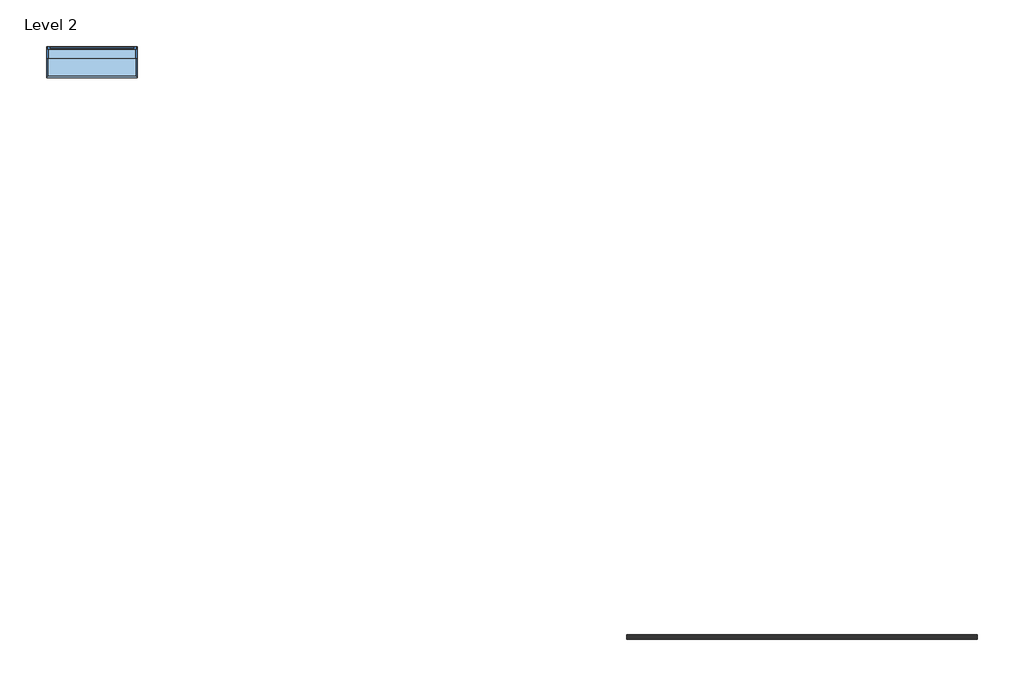
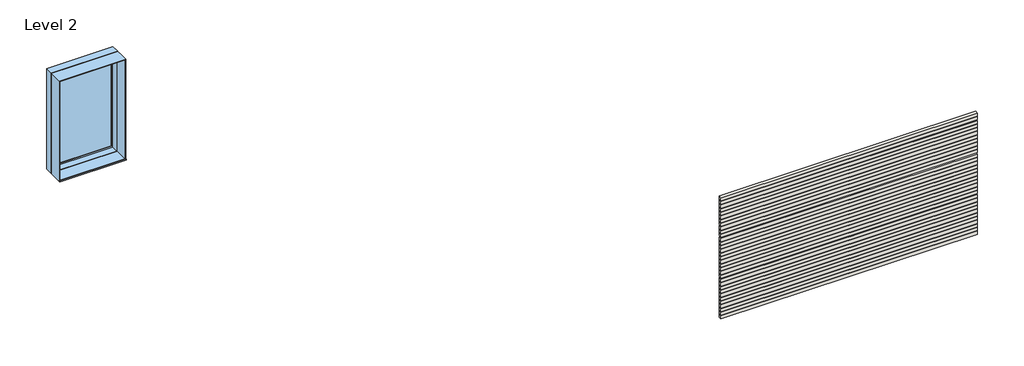
# One storey: 3 walls, 1 window.
"""IFC4 building model written with IfcOpenShell, lengths in millimetres."""

from ifc_helpers import new_model, si_unit, frame, origin, place, context, project, spatial, polyline, outline, extrude, transform, mapped, element, save
from components import window_e9f06afb

model = new_model("IFC4")

# Units and contexts
model_context = context("Model", 3, world=origin())
ifc_project = project(units=[si_unit("LENGTHUNIT", "METRE", prefix="MILLI")], contexts=[model_context])

# Site, building, storey
site = spatial("IfcSite", under=ifc_project)
building = spatial("IfcBuilding", under=site)
storey = spatial("IfcBuildingStorey", under=building, Name="Level 2", Elevation=3048.0)

# Walls
placement = place(None, origin())
element("IfcWall", 1, ObjectType="Generic - 3\" white 2", at=placement, inside=storey, context=model_context, shape_type="SweptSolid", body=[
    extrude(outline(polyline([(7352.8964234, 5106.5999244), (1468.8829427, 5106.5999244), (1468.8829427, 5182.7999244), (7352.8964234, 5182.7999244), (7352.8964234, 5106.5999244)])), frame((0.0, 0.0, 1971.675), z_axis=(0.0, 0.0, 1.0), x_axis=(1.0, 0.0, 0.0)), (0.0, 0.0, 1.0), 76.2),
    extrude(outline(polyline([(7352.8964234, 5106.5999244), (1468.8829427, 5106.5999244), (1468.8829427, 5182.7999244), (7352.8964234, 5182.7999244), (7352.8964234, 5106.5999244)])), frame((0.0, 0.0, 2060.575), z_axis=(0.0, 0.0, 1.0), x_axis=(1.0, 0.0, 0.0)), (0.0, 0.0, 1.0), 76.2),
    extrude(outline(polyline([(7352.8964234, 5106.5999244), (1468.8829427, 5106.5999244), (1468.8829427, 5182.7999244), (7352.8964234, 5182.7999244), (7352.8964234, 5106.5999244)])), frame((0.0, 0.0, 2149.475), z_axis=(0.0, 0.0, 1.0), x_axis=(1.0, 0.0, 0.0)), (0.0, 0.0, 1.0), 76.2),
    extrude(outline(polyline([(7352.8964234, 5106.5999244), (1468.8829427, 5106.5999244), (1468.8829427, 5182.7999244), (7352.8964234, 5182.7999244), (7352.8964234, 5106.5999244)])), frame((0.0, 0.0, 2238.375), z_axis=(0.0, 0.0, 1.0), x_axis=(1.0, 0.0, 0.0)), (0.0, 0.0, 1.0), 76.2),
    extrude(outline(polyline([(7352.8964234, 5106.5999244), (1468.8829427, 5106.5999244), (1468.8829427, 5182.7999244), (7352.8964234, 5182.7999244), (7352.8964234, 5106.5999244)])), frame((0.0, 0.0, 2327.275), z_axis=(0.0, 0.0, 1.0), x_axis=(1.0, 0.0, 0.0)), (0.0, 0.0, 1.0), 76.2),
    extrude(outline(polyline([(7352.8964234, 5106.5999244), (1468.8829427, 5106.5999244), (1468.8829427, 5182.7999244), (7352.8964234, 5182.7999244), (7352.8964234, 5106.5999244)])), frame((0.0, 0.0, 2416.175), z_axis=(0.0, 0.0, 1.0), x_axis=(1.0, 0.0, 0.0)), (0.0, 0.0, 1.0), 76.2),
    extrude(outline(polyline([(7352.8964234, 5106.5999244), (1468.8829427, 5106.5999244), (1468.8829427, 5182.7999244), (7352.8964234, 5182.7999244), (7352.8964234, 5106.5999244)])), frame((0.0, 0.0, 2505.075), z_axis=(0.0, 0.0, 1.0), x_axis=(1.0, 0.0, 0.0)), (0.0, 0.0, 1.0), 76.2),
    extrude(outline(polyline([(7352.8964234, 5106.5999244), (1468.8829427, 5106.5999244), (1468.8829427, 5182.7999244), (7352.8964234, 5182.7999244), (7352.8964234, 5106.5999244)])), frame((0.0, 0.0, 2593.975), z_axis=(0.0, 0.0, 1.0), x_axis=(1.0, 0.0, 0.0)), (0.0, 0.0, 1.0), 76.2),
    extrude(outline(polyline([(7352.8964234, 5106.5999244), (1468.8829427, 5106.5999244), (1468.8829427, 5182.7999244), (7352.8964234, 5182.7999244), (7352.8964234, 5106.5999244)])), frame((0.0, 0.0, 2682.875), z_axis=(0.0, 0.0, 1.0), x_axis=(1.0, 0.0, 0.0)), (0.0, 0.0, 1.0), 76.2),
    extrude(outline(polyline([(7352.8964234, 5106.5999244), (1468.8829427, 5106.5999244), (1468.8829427, 5182.7999244), (7352.8964234, 5182.7999244), (7352.8964234, 5106.5999244)])), frame((0.0, 0.0, 2771.775), z_axis=(0.0, 0.0, 1.0), x_axis=(1.0, 0.0, 0.0)), (0.0, 0.0, 1.0), 76.2),
    extrude(outline(polyline([(7352.8964234, 5106.5999244), (1468.8829427, 5106.5999244), (1468.8829427, 5182.7999244), (7352.8964234, 5182.7999244), (7352.8964234, 5106.5999244)])), frame((0.0, 0.0, 2860.675), z_axis=(0.0, 0.0, 1.0), x_axis=(1.0, 0.0, 0.0)), (0.0, 0.0, 1.0), 76.2),
])
element("IfcWall", 2, ObjectType="Generic - 3\" white 2", at=placement, inside=storey, context=model_context, shape_type="SweptSolid", body=[
    extrude(outline(polyline([(7352.8964234, 5106.5999244), (1468.8829427, 5106.5999244), (1468.8829427, 5182.7999244), (7352.8964234, 5182.7999244), (7352.8964234, 5106.5999244)])), frame((0.0, 0.0, 2959.1), z_axis=(0.0, 0.0, 1.0), x_axis=(1.0, 0.0, 0.0)), (0.0, 0.0, 1.0), 76.2),
    extrude(outline(polyline([(7352.8964234, 5106.5999244), (1468.8829427, 5106.5999244), (1468.8829427, 5182.7999244), (7352.8964234, 5182.7999244), (7352.8964234, 5106.5999244)])), frame((0.0, 0.0, 3048.0), z_axis=(0.0, 0.0, 1.0), x_axis=(1.0, 0.0, 0.0)), (0.0, 0.0, 1.0), 76.2),
    extrude(outline(polyline([(7352.8964234, 5106.5999244), (1468.8829427, 5106.5999244), (1468.8829427, 5182.7999244), (7352.8964234, 5182.7999244), (7352.8964234, 5106.5999244)])), frame((0.0, 0.0, 3136.9), z_axis=(0.0, 0.0, 1.0), x_axis=(1.0, 0.0, 0.0)), (0.0, 0.0, 1.0), 76.2),
    extrude(outline(polyline([(7352.8964234, 5106.5999244), (1468.8829427, 5106.5999244), (1468.8829427, 5182.7999244), (7352.8964234, 5182.7999244), (7352.8964234, 5106.5999244)])), frame((0.0, 0.0, 3225.8), z_axis=(0.0, 0.0, 1.0), x_axis=(1.0, 0.0, 0.0)), (0.0, 0.0, 1.0), 76.2),
    extrude(outline(polyline([(7352.8964234, 5106.5999244), (1468.8829427, 5106.5999244), (1468.8829427, 5182.7999244), (7352.8964234, 5182.7999244), (7352.8964234, 5106.5999244)])), frame((0.0, 0.0, 3314.7), z_axis=(0.0, 0.0, 1.0), x_axis=(1.0, 0.0, 0.0)), (0.0, 0.0, 1.0), 76.2),
    extrude(outline(polyline([(7352.8964234, 5106.5999244), (1468.8829427, 5106.5999244), (1468.8829427, 5182.7999244), (7352.8964234, 5182.7999244), (7352.8964234, 5106.5999244)])), frame((0.0, 0.0, 3403.6), z_axis=(0.0, 0.0, 1.0), x_axis=(1.0, 0.0, 0.0)), (0.0, 0.0, 1.0), 76.2),
    extrude(outline(polyline([(7352.8964234, 5106.5999244), (1468.8829427, 5106.5999244), (1468.8829427, 5182.7999244), (7352.8964234, 5182.7999244), (7352.8964234, 5106.5999244)])), frame((0.0, 0.0, 3492.5), z_axis=(0.0, 0.0, 1.0), x_axis=(1.0, 0.0, 0.0)), (0.0, 0.0, 1.0), 76.2),
    extrude(outline(polyline([(7352.8964234, 5106.5999244), (1468.8829427, 5106.5999244), (1468.8829427, 5182.7999244), (7352.8964234, 5182.7999244), (7352.8964234, 5106.5999244)])), frame((0.0, 0.0, 3581.4), z_axis=(0.0, 0.0, 1.0), x_axis=(1.0, 0.0, 0.0)), (0.0, 0.0, 1.0), 76.2),
    extrude(outline(polyline([(7352.8964234, 5106.5999244), (1468.8829427, 5106.5999244), (1468.8829427, 5182.7999244), (7352.8964234, 5182.7999244), (7352.8964234, 5106.5999244)])), frame((0.0, 0.0, 3670.3), z_axis=(0.0, 0.0, 1.0), x_axis=(1.0, 0.0, 0.0)), (0.0, 0.0, 1.0), 76.2),
    extrude(outline(polyline([(7352.8964234, 5106.5999244), (1468.8829427, 5106.5999244), (1468.8829427, 5182.7999244), (7352.8964234, 5182.7999244), (7352.8964234, 5106.5999244)])), frame((0.0, 0.0, 3759.2), z_axis=(0.0, 0.0, 1.0), x_axis=(1.0, 0.0, 0.0)), (0.0, 0.0, 1.0), 76.2),
    extrude(outline(polyline([(7352.8964234, 5106.5999244), (1468.8829427, 5106.5999244), (1468.8829427, 5182.7999244), (7352.8964234, 5182.7999244), (7352.8964234, 5106.5999244)])), frame((0.0, 0.0, 3848.1), z_axis=(0.0, 0.0, 1.0), x_axis=(1.0, 0.0, 0.0)), (0.0, 0.0, 1.0), 76.2),
])
element("IfcWall", 3, ObjectType="Generic - 3\" white 2", at=placement, inside=storey, context=model_context, shape_type="SweptSolid", body=[
    extrude(outline(polyline([(7352.8964234, 5106.5999244), (1468.8829427, 5106.5999244), (1468.8829427, 5182.7999244), (7352.8964234, 5182.7999244), (7352.8964234, 5106.5999244)])), frame((0.0, 0.0, 3950.7840126), z_axis=(0.0, 0.0, 1.0), x_axis=(1.0, 0.0, 0.0)), (0.0, 0.0, 1.0), 76.2),
    extrude(outline(polyline([(7352.8964234, 5106.5999244), (1468.8829427, 5106.5999244), (1468.8829427, 5182.7999244), (7352.8964234, 5182.7999244), (7352.8964234, 5106.5999244)])), frame((0.0, 0.0, 4039.6840126), z_axis=(0.0, 0.0, 1.0), x_axis=(1.0, 0.0, 0.0)), (0.0, 0.0, 1.0), 76.2),
    extrude(outline(polyline([(7352.8964234, 5106.5999244), (1468.8829427, 5106.5999244), (1468.8829427, 5182.7999244), (7352.8964234, 5182.7999244), (7352.8964234, 5106.5999244)])), frame((0.0, 0.0, 4128.5840126), z_axis=(0.0, 0.0, 1.0), x_axis=(1.0, 0.0, 0.0)), (0.0, 0.0, 1.0), 76.2),
    extrude(outline(polyline([(7352.8964234, 5106.5999244), (1468.8829427, 5106.5999244), (1468.8829427, 5182.7999244), (7352.8964234, 5182.7999244), (7352.8964234, 5106.5999244)])), frame((0.0, 0.0, 4217.4840126), z_axis=(0.0, 0.0, 1.0), x_axis=(1.0, 0.0, 0.0)), (0.0, 0.0, 1.0), 76.2),
    extrude(outline(polyline([(7352.8964234, 5106.5999244), (1468.8829427, 5106.5999244), (1468.8829427, 5182.7999244), (7352.8964234, 5182.7999244), (7352.8964234, 5106.5999244)])), frame((0.0, 0.0, 4306.3840126), z_axis=(0.0, 0.0, 1.0), x_axis=(1.0, 0.0, 0.0)), (0.0, 0.0, 1.0), 76.2),
    extrude(outline(polyline([(7352.8964234, 5106.5999244), (1468.8829427, 5106.5999244), (1468.8829427, 5182.7999244), (7352.8964234, 5182.7999244), (7352.8964234, 5106.5999244)])), frame((0.0, 0.0, 4395.2840126), z_axis=(0.0, 0.0, 1.0), x_axis=(1.0, 0.0, 0.0)), (0.0, 0.0, 1.0), 76.2),
    extrude(outline(polyline([(7352.8964234, 5106.5999244), (1468.8829427, 5106.5999244), (1468.8829427, 5182.7999244), (7352.8964234, 5182.7999244), (7352.8964234, 5106.5999244)])), frame((0.0, 0.0, 4484.1840126), z_axis=(0.0, 0.0, 1.0), x_axis=(1.0, 0.0, 0.0)), (0.0, 0.0, 1.0), 76.2),
    extrude(outline(polyline([(7352.8964234, 5106.5999244), (1468.8829427, 5106.5999244), (1468.8829427, 5182.7999244), (7352.8964234, 5182.7999244), (7352.8964234, 5106.5999244)])), frame((0.0, 0.0, 4573.0840126), z_axis=(0.0, 0.0, 1.0), x_axis=(1.0, 0.0, 0.0)), (0.0, 0.0, 1.0), 76.2),
    extrude(outline(polyline([(7352.8964234, 5106.5999244), (1468.8829427, 5106.5999244), (1468.8829427, 5182.7999244), (7352.8964234, 5182.7999244), (7352.8964234, 5106.5999244)])), frame((0.0, 0.0, 4661.9840126), z_axis=(0.0, 0.0, 1.0), x_axis=(1.0, 0.0, 0.0)), (0.0, 0.0, 1.0), 76.2),
    extrude(outline(polyline([(7352.8964234, 5106.5999244), (1468.8829427, 5106.5999244), (1468.8829427, 5182.7999244), (7352.8964234, 5182.7999244), (7352.8964234, 5106.5999244)])), frame((0.0, 0.0, 4750.8840126), z_axis=(0.0, 0.0, 1.0), x_axis=(1.0, 0.0, 0.0)), (0.0, 0.0, 1.0), 76.2),
    extrude(outline(polyline([(7352.8964234, 5106.5999244), (1468.8829427, 5106.5999244), (1468.8829427, 5182.7999244), (7352.8964234, 5182.7999244), (7352.8964234, 5106.5999244)])), frame((0.0, 0.0, 4839.7840126), z_axis=(0.0, 0.0, 1.0), x_axis=(1.0, 0.0, 0.0)), (0.0, 0.0, 1.0), 76.2),
])

# Window
window_shape = window_e9f06afb(model_context)
element("IfcWindow", 4, ObjectType="Instance - Fixed.0001 : 60\" x 96\"", at=placement, inside=storey, context=model_context, shape_type="MappedRepresentation", body=[
    mapped(window_shape, transform((-7538.8964397, 14701.2629979, 2387.6), x_axis=(-1.0, 0.0, 0.0), y_axis=(0.0, -1.0, 0.0), z_axis=(0.0, 0.0, 1.0))),
])

save(model, "model.ifc")

# Revit data of these elements
# Type "Generic - 3\" white 2"
#   Assembly Code = "B2010"
#   Layers, outside or top first: 0' - 3" "Door - Frame" (function 1)
# Type "Instance - Fixed.0001 : 60\" x 96\""
#   Type Mark = "13"
#   Construction Type Id = "MDOOR"
#   Assembly Code = "B2020100"
#   Analytic Construction = "Metal"
#   Heat Transfer Coefficient (U) = 0.651978 BTU/(h·ft²·°F)
#   Height [instance default] = 6' - 0"
#   Default Sill Height = 2' - 0"
#   Width [instance default] = 3' - 0"
#   Window Inset = 1' - 6"
#   Define Thermal Properties by = 1
#   Glass Pane Material = Glass
#   Sash Material = Door - Frame
#   Visual Light Transmittance = 0
#   Thermal Resistance (R) = 0
#   Solar Heat Gain Coefficient = 0
#   Wall Closure = (empty or 0)
# Element 1 (IfcWall, "Generic - 3\" white 2")
#   built-in parameter 1001111 = -3' - 6 3/8"
#   Top Offset = 0' - 0"
#   Base Offset = -3' - 6 3/8"
#   Unconnected Height = 3' - 2.29268"
#   wall height = 3' - 2.29268"
#   Phase Created = New Construction
#   Base Constraint = Level 2
#   Materials on its faces: "Door - Frame"
# Element 2 (IfcWall, "Generic - 3\" white 2")
#   built-in parameter 1001111 = -0' - 3 1/2"
#   Top Offset = 0' - 0"
#   Base Offset = -0' - 3 1/2"
#   Unconnected Height = 3' - 2.29268"
#   wall height = 3' - 2.29268"
#   Phase Created = New Construction
#   Base Constraint = Level 2
#   Materials on its faces: "Door - Frame"
# Element 3 (IfcWall, "Generic - 3\" white 2")
#   built-in parameter 1001111 = 2' - 11.54268"
#   Top Offset = 0' - 0"
#   Base Offset = 2' - 11.54268"
#   Unconnected Height = 3' - 2.29268"
#   wall height = 3' - 2.29268"
#   Phase Created = New Construction
#   Base Constraint = Level 2
#   Materials on its faces: "Door - Frame"
# Element 4 (IfcWindow, "Instance - Fixed.0001 : 60\" x 96\"")
#   Mark = "1"
#   Width = 5' - 0"
#   Height = 8' - 0"
#   Phase Created = New Construction
#   Materials on its faces: "Door - Frame", "Glass"
# Materials
#   "Door - Frame": colour RGB 118 70 51, transparency 0, Cost = 0
#   "Glass": class "Glass", colour RGB 0 128 192, transparency 0.75, Description = "Soda Lime Glass", Cost = 0
